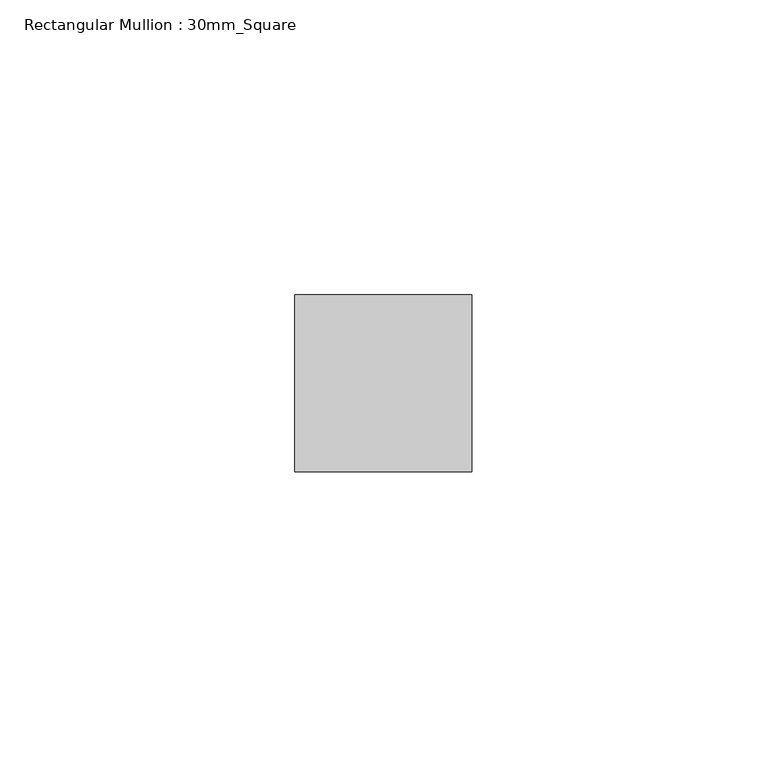
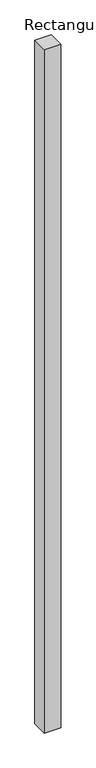
"""IFC4 building model written with IfcOpenShell, lengths in millimetres: member geometry, Rectangular Mullion : 30mm_Square."""

from ifc_helpers import new_model, si_unit, frame, origin, place, context, project, spatial, polyline, outline, extrude, source, transform, mapped, element, save


def rectangular_mullion_30mm_square_4b249e81(model_context):
    return source(origin(), model_context, "Body", "SweptSolid", [
        extrude(outline(polyline([(0.0, 15.0), (0.0, -15.0), (-30.0, -15.0), (-30.0, 15.0), (0.0, 15.0)])), frame((0.0, 0.0, -1330.8429687), z_axis=(0.0, 0.0, 1.0), x_axis=(1.0, 0.0, 0.0)), (0.0, 0.0, 1.0), 1330.8429687),
    ])


if __name__ == "__main__":
    model = new_model("IFC4")
    model_context = context("Model", 3, world=origin())
    ifc_project = project(units=[si_unit("LENGTHUNIT", "METRE", prefix="MILLI")], contexts=[model_context])
    site = spatial("IfcSite", under=ifc_project)
    building = spatial("IfcBuilding", under=site)
    placement = place(None, origin())
    rectangular_mullion_30mm_square_shape = rectangular_mullion_30mm_square_4b249e81(model_context)
    element("IfcMember", 1, ObjectType="Rectangular Mullion : 30mm_Square", at=placement, inside=building, context=model_context, shape_type="MappedRepresentation", body=[
        mapped(rectangular_mullion_30mm_square_shape, transform((0.0, 0.0, 0.0), x_axis=(1.0, 0.0, 0.0), y_axis=(0.0, 1.0, 0.0), z_axis=(0.0, 0.0, 1.0))),
    ])
    save(model, "model.ifc")

# Revit data of these elements
# Type "Rectangular Mullion : 30mm_Square"
#   Keynote = "H11"
#   built-in parameter 1007304 = 0.0984252 (stored number, unit not read)
#   built-in parameter 1007301 = 0.0492126 (stored number, unit not read)
#   built-in parameter 1007300 = 0.0492126 (stored number, unit not read)
# Element 1 (IfcMember, "Rectangular Mullion : 30mm_Square")
#   Materials on its faces: "Aluminium"
# Materials
#   "Aluminium": class "Metal", colour RGB 247 247 247, transparency 0, Description = "Aluminium 6061", Cost = 0
